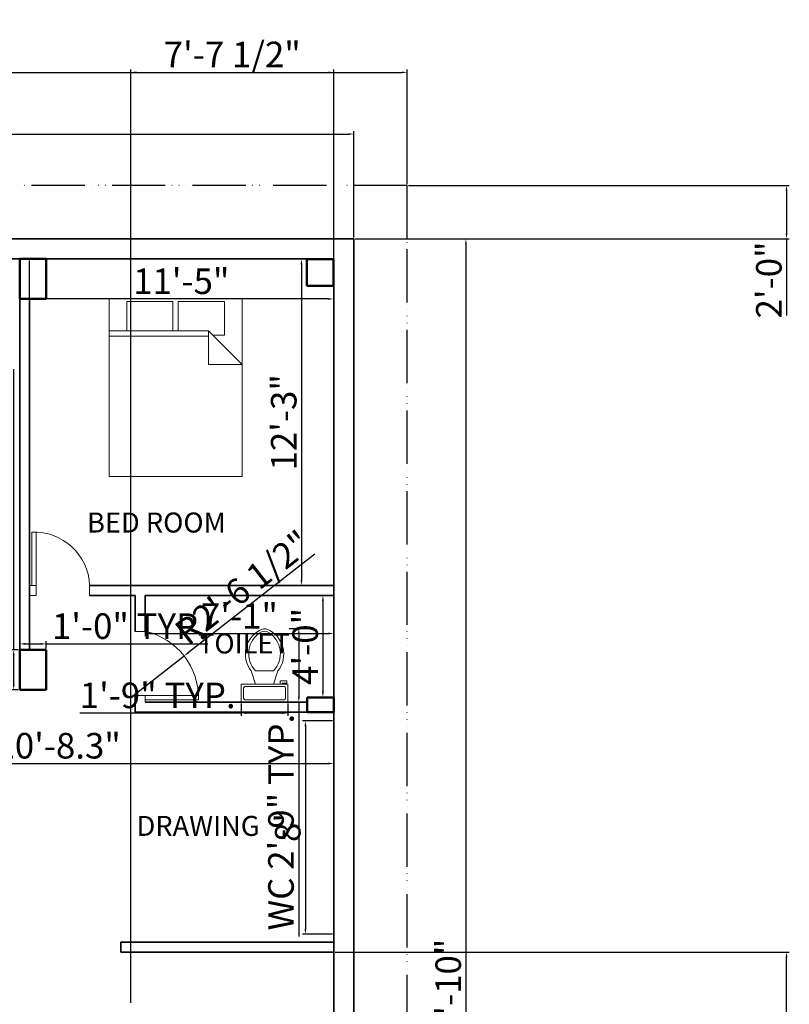
# Model space of a CAD drawing. Units: inches. Extents: x 2680 to 3617, y 1720 to 2823.
# Tile 4 of 4: x 3270 to 3617, y 2380 to 2823. Entities that reach past the tile are written whole.
import ezdxf

# ---------------------------------------------------------------- set-up
doc = ezdxf.new("R2010")
doc.units = ezdxf.units.IN
doc.linetypes.add('ACAD_ISO06W100', pattern=[36, 24, -3, 0, -3, 0, -3, 0, -3])
for name, color, linetype, lineweight in [('A-ANNO-DIMS', 2, 'Continuous', 18), ('A-AREA-IDEN', 244, 'Continuous', 18), ('A-COLS', 1, 'Continuous', 50), ('A-DOOR', 4, 'Continuous', 18), ('A-FLOR-FIXT', 9, 'Continuous', 18), ('A-FURN', 8, 'Continuous', 18), ('A-WALL', 7, 'Continuous', 35), ('C-PROP', 6, 'ACAD_ISO06W100', 25)]:
    doc.layers.add(name, color=color, linetype=linetype, lineweight=lineweight)
doc.styles.get("Standard").update_dxf_attribs({"font": 'arial.ttf'})
doc.dimstyles.new('ISO-25', dxfattribs={"dimtxt": 11.5, "dimasz": 2.5, "dimexe": 1.25, "dimexo": 0.625, "dimtad": 1, "dimdec": 1, "dimlunit": 3, "dimtxsty": 'Standard', "dimcen": 2.5, "dimadec": 0, "dimazin": 0, "dimtfac": 1, "dimtdec": 1, "dimtmove": 0, "dimatfit": 3, "dimfxl": 1, "dimarcsym": 0})

# ---------------------------------------------------------------- blocks, each defined once
blk = doc.blocks.new('*D8')
at = {"layer": 'A-ANNO-DIMS', "color": 0, "lineweight": -2, "transparency": 16777216}
for p, q in [((3274.67, 2714.72), (3274.67, 2696.18)), ((3411.72, 2714.72), (3411.72, 2696.18)), ((3409.22, 2697.43), (3277.17, 2697.43))]:
    blk.add_line(p, q, dxfattribs=at)
at = {"layer": 'A-ANNO-DIMS', "color": 0, "lineweight": 70, "transparency": 16777216}
for points in [[(3277.17, 2697.84), (3277.17, 2697.01), (3274.67, 2697.43)], [(3409.22, 2697.84), (3409.22, 2697.01), (3411.72, 2697.43)]]:
    blk.add_solid(points, dxfattribs=at)
at = {"layer": 'Defpoints', "color": 0, "lineweight": 70, "transparency": 16777216}
for p in [(3274.67, 2715.35), (3411.72, 2715.35), (3274.67, 2697.43)]:
    blk.add_point(p, dxfattribs=at)
at = {"layer": 'A-ANNO-DIMS', "color": 0, "transparency": 16777216, "insert": (3343.2, 2703.92), "char_height": 11.5, "attachment_point": 5}
blk.add_mtext('11\'-5"', dxfattribs=at)
blk = doc.blocks.new('*D9')
at = {"layer": 'A-ANNO-DIMS', "color": 0, "lineweight": -2, "transparency": 16777216}
for p, q in [((3411.29, 2715.35), (3396.09, 2715.35)), ((3397.34, 2712.85), (3397.34, 2571)), ((3411.29, 2568.5), (3396.09, 2568.5))]:
    blk.add_line(p, q, dxfattribs=at)
at = {"layer": 'A-ANNO-DIMS', "color": 0, "lineweight": 70, "transparency": 16777216}
for points in [[(3396.92, 2712.85), (3397.76, 2712.85), (3397.34, 2715.35)], [(3396.92, 2571), (3397.76, 2571), (3397.34, 2568.5)]]:
    blk.add_solid(points, dxfattribs=at)
at = {"layer": 'Defpoints', "color": 0, "lineweight": 70, "transparency": 16777216}
for p in [(3411.91, 2715.35), (3397.34, 2568.5), (3411.91, 2568.5)]:
    blk.add_point(p, dxfattribs=at)
at = {"layer": 'A-ANNO-DIMS', "color": 0, "transparency": 16777216, "insert": (3390.84, 2641.93), "char_height": 11.5, "attachment_point": 5, "rotation": 90}
blk.add_mtext('12\'-3"', dxfattribs=at)
blk = doc.blocks.new('*D12')
at = {"layer": 'A-ANNO-DIMS', "color": 0, "lineweight": -2, "transparency": 16777216}
for p, q in [((3326.91, 2563.38), (3326.91, 2545.63)), ((3411.91, 2563.38), (3411.91, 2545.63)), ((3329.41, 2546.88), (3409.41, 2546.88))]:
    blk.add_line(p, q, dxfattribs=at)
at = {"layer": 'A-ANNO-DIMS', "color": 0, "lineweight": 70, "transparency": 16777216}
for points in [[(3329.41, 2547.3), (3329.41, 2546.47), (3326.91, 2546.88)], [(3409.41, 2547.3), (3409.41, 2546.47), (3411.91, 2546.88)]]:
    blk.add_solid(points, dxfattribs=at)
at = {"layer": 'Defpoints', "color": 0, "lineweight": 70, "transparency": 16777216}
for p in [(3326.91, 2564), (3411.91, 2564), (3411.91, 2546.88)]:
    blk.add_point(p, dxfattribs=at)
at = {"layer": 'A-ANNO-DIMS', "color": 0, "transparency": 16777216, "insert": (3369.41, 2553.28), "char_height": 11.5, "attachment_point": 5}
blk.add_mtext('7\'-1"', dxfattribs=at)
blk = doc.blocks.new('*D13')
at = {"layer": 'A-ANNO-DIMS', "color": 0, "lineweight": -2, "transparency": 16777216}
for p, q in [((3411.29, 2564), (3405.73, 2564)), ((3406.98, 2561.5), (3406.98, 2520.65)), ((3411.29, 2518.15), (3405.73, 2518.15))]:
    blk.add_line(p, q, dxfattribs=at)
at = {"layer": 'A-ANNO-DIMS', "color": 0, "lineweight": 70, "transparency": 16777216}
for points in [[(3406.56, 2561.5), (3407.4, 2561.5), (3406.98, 2564)], [(3406.56, 2520.65), (3407.4, 2520.65), (3406.98, 2518.15)]]:
    blk.add_solid(points, dxfattribs=at)
at = {"layer": 'Defpoints', "color": 0, "lineweight": 70, "transparency": 16777216}
for p in [(3411.91, 2564), (3406.98, 2518.15), (3411.91, 2518.15)]:
    blk.add_point(p, dxfattribs=at)
at = {"layer": 'A-ANNO-DIMS', "color": 0, "transparency": 16777216, "insert": (3400.48, 2541.08), "char_height": 11.5, "attachment_point": 5, "rotation": 90}
blk.add_mtext('4\'-0"', dxfattribs=at)
blk = doc.blocks.new('*D14')
at = {"layer": 'A-ANNO-DIMS', "color": 0, "lineweight": -2, "transparency": 16777216}
for p, q in [((3411.29, 2507.58), (3397.87, 2507.58)), ((3399.12, 2505.08), (3399.12, 2414.04)), ((3411.29, 2411.54), (3397.87, 2411.54))]:
    blk.add_line(p, q, dxfattribs=at)
at = {"layer": 'A-ANNO-DIMS', "color": 0, "lineweight": 70, "transparency": 16777216}
for points in [[(3398.71, 2505.08), (3399.54, 2505.08), (3399.12, 2507.58)], [(3398.71, 2414.04), (3399.54, 2414.04), (3399.12, 2411.54)]]:
    blk.add_solid(points, dxfattribs=at)
at = {"layer": 'Defpoints', "color": 0, "lineweight": 70, "transparency": 16777216}
for p in [(3411.91, 2507.58), (3399.12, 2411.54), (3411.91, 2411.54)]:
    blk.add_point(p, dxfattribs=at)
at = {"layer": 'A-ANNO-DIMS', "color": 0, "transparency": 16777216, "insert": (3392.63, 2459.56), "char_height": 11.5, "attachment_point": 5, "rotation": 90}
blk.add_mtext("8'", dxfattribs=at)
blk = doc.blocks.new('*D27')
at = {"layer": 'A-ANNO-DIMS', "color": 0, "lineweight": -2, "transparency": 16777216}
for p, q in [((3163.61, 2520.88), (3163.61, 2487.12)), ((3411.91, 2517.52), (3411.91, 2487.12)), ((3166.11, 2488.37), (3409.41, 2488.37))]:
    blk.add_line(p, q, dxfattribs=at)
at = {"layer": 'A-ANNO-DIMS', "color": 0, "lineweight": 70, "transparency": 16777216}
for points in [[(3166.11, 2488.78), (3166.11, 2487.95), (3163.61, 2488.37)], [(3409.41, 2488.78), (3409.41, 2487.95), (3411.91, 2488.37)]]:
    blk.add_solid(points, dxfattribs=at)
at = {"layer": 'Defpoints', "color": 0, "lineweight": 70, "transparency": 16777216}
for p in [(3163.61, 2521.5), (3411.91, 2518.15), (3411.91, 2488.37)]:
    blk.add_point(p, dxfattribs=at)
at = {"layer": 'A-ANNO-DIMS', "color": 0, "transparency": 16777216, "insert": (3287.76, 2494.87), "char_height": 11.5, "attachment_point": 5}
blk.add_mtext('20\'-8.3"', dxfattribs=at)
blk = doc.blocks.new('*D41')
at = {"layer": 'A-ANNO-DIMS', "color": 0, "lineweight": -2, "transparency": 16777216}
for p, q in [((2888.91, 2725.13), (2888.91, 2772.91)), ((2891.41, 2771.66), (3418.41, 2771.66)), ((3420.91, 2725.13), (3420.91, 2772.91))]:
    blk.add_line(p, q, dxfattribs=at)
at = {"layer": 'A-ANNO-DIMS', "color": 0, "lineweight": 70, "transparency": 16777216}
for points in [[(2891.41, 2772.07), (2891.41, 2771.24), (2888.91, 2771.66)], [(3418.41, 2772.07), (3418.41, 2771.24), (3420.91, 2771.66)]]:
    blk.add_solid(points, dxfattribs=at)
at = {"layer": 'Defpoints', "color": 0, "lineweight": 70, "transparency": 16777216}
for p in [(3420.91, 2771.66), (2888.91, 2724.5), (3420.91, 2724.5)]:
    blk.add_point(p, dxfattribs=at)
at = {"layer": 'A-ANNO-DIMS', "color": 0, "transparency": 16777216, "insert": (3154.91, 2778.03), "char_height": 11.5, "attachment_point": 5}
blk.add_mtext('44\'-4"', dxfattribs=at)
blk = doc.blocks.new('*D43')
at = {"layer": 'A-ANNO-DIMS', "color": 0, "lineweight": -2, "transparency": 16777216}
for p, q in [((3421.54, 2724.5), (3472.64, 2724.5)), ((3471.39, 2722), (3471.39, 2045)), ((3421.54, 2042.5), (3472.64, 2042.5))]:
    blk.add_line(p, q, dxfattribs=at)
at = {"layer": 'A-ANNO-DIMS', "color": 0, "lineweight": 70, "transparency": 16777216}
for points in [[(3470.98, 2722), (3471.81, 2722), (3471.39, 2724.5)], [(3470.98, 2045), (3471.81, 2045), (3471.39, 2042.5)]]:
    blk.add_solid(points, dxfattribs=at)
at = {"layer": 'Defpoints', "color": 0, "lineweight": 70, "transparency": 16777216}
for p in [(3420.91, 2724.5), (3420.91, 2042.5), (3471.39, 2042.5)]:
    blk.add_point(p, dxfattribs=at)
at = {"layer": 'A-ANNO-DIMS', "color": 0, "transparency": 16777216, "insert": (3464.9, 2383.5), "char_height": 11.5, "attachment_point": 5, "rotation": 90}
blk.add_mtext('56\'-10"', dxfattribs=at)
blk = doc.blocks.new('Bed - Queen')
for p, q in [((0, -80.00003), (0, 0)), ((0, 0), (59.99999, 0)), ((59.99999, 0), (59.99999, -80.00003)), ((7.99999, -1.2), (28.79998, -1.2)), ((7.99999, -14.4), (7.99999, -1.2)), ((28.79998, -1.2), (28.79998, -14.4)), ((31.19999, -1.2), (51.99999, -1.2)), ((31.19999, -14.4), (31.19999, -1.2)), ((51.99999, -1.2), (51.99999, -16.4)), ((0, -14.4), (44.8, -14.4)), ((44.8, -16.8), (0, -16.8)), ((59.99999, -29.6), (44.8, -14.4)), ((44.8, -14.4), (44.8, -29.6)), ((51.99999, -16.4), (46.79936, -16.4)), ((44.8, -29.6), (59.99999, -29.6)), ((59.99999, -80.00003), (0, -80.00003))]:
    blk.add_line(p, q)
blk = doc.blocks.new('Toilet - top')
for p, q in [((9.5, -6), (9.5, -2)), ((-10, -8.5), (-8, -8.5)), ((-10, -9.5), (-10, -8.5)), ((-8, -8.5), (-8, -8)), ((-7, -8), (-7, -9.5)), ((-4, -8), (-6, -14)), ((4, -8), (6, -14)), ((-7, -9.5), (-10, -9.5)), ((4, -14), (-4, -14))]:
    blk.add_line(p, q)
blk.add_lwpolyline([(10.5, -8), (10.5, 0), (-10.5, 0), (-10.5, -8)], close=True)
for points in [[(-9.5, -2), (-9.5, -6)], [(8.5, -1), (-8.5, -1)], [(-8.5, -7), (8.5, -7)]]:
    blk.add_lwpolyline(points)
for centre, radius, start, end in [((-8.62, -1.88), 0.884, 81.8699, 188.1301), ((8.62, -1.88), 0.884, 351.8699, 98.1301), ((-8.62, -6.12), 0.884, 171.8699, 278.1301), ((8.62, -6.12), 0.884, 261.8699, 8.1301), ((3.52, -21.58), 12.17, 141.4691, 247.9714), ((4.2, -21.82), 11.33, 136.3677, 238.9468), ((-3.52, -21.58), 12.17, 292.0284, 38.5307), ((-4.2, -21.82), 11.33, 301.053, 43.6321), ((0, -27.88), 4, 245.7318, 294.2682), ((0, -29), 4, 254.8605, 285.1395)]:
    blk.add_arc(centre, radius, start, end)
blk = doc.blocks.new('COL-12X6P64')
for p, q in [((0, 0), (0, 6.64)), ((0, 6.64), (12, 6.64)), ((12, 6.64), (12, 0)), ((12, 0), (0, 0))]:
    blk.add_line(p, q)
blk = doc.blocks.new('COL-12X18')
for p, q in [((0, 0), (0, 18)), ((0, 18), (12, 18)), ((12, 18), (12, 0)), ((12, 18), (12, 0)), ((12, 0), (0, 0))]:
    blk.add_line(p, q)
blk = doc.blocks.new('COL-12X12')
for p, q in [((0, 12), (12, 12)), ((0, 0), (0, 12)), ((12, 12), (12, 0)), ((12, 0), (0, 0))]:
    blk.add_line(p, q)
blk = doc.blocks.new('DOOR-SINGLE-27')
for p, q in [((26, 28.5), (24, 28.5)), ((24, 28.5), (24, 0)), ((26, 4.5), (26, 28.5)), ((0, 4.5), (0, 0)), ((24, 4.5), (27, 4.5)), ((27, 4.5), (26, 4.5)), ((24, 0), (27, 0))]:
    blk.add_line(p, q)
blk.add_arc((25, 3.5), 25.02, 87.7094, 177.7094)
blk = doc.blocks.new('*D56')
at = {"layer": 'A-ANNO-DIMS', "color": 0, "lineweight": -2, "transparency": 16777216}
for p, q in [((3391.83, 2549.05), (3397.41, 2549.05)), ((3396.16, 2546.55), (3396.16, 2518.5)), ((3391.83, 2516), (3397.41, 2516)), ((3396.16, 2516), (3396.16, 2410.46))]:
    blk.add_line(p, q, dxfattribs=at)
at = {"layer": 'A-ANNO-DIMS', "color": 0, "lineweight": 70, "transparency": 16777216}
for points in [[(3395.74, 2546.55), (3396.58, 2546.55), (3396.16, 2549.05)], [(3395.74, 2518.5), (3396.58, 2518.5), (3396.16, 2516)]]:
    blk.add_solid(points, dxfattribs=at)
at = {"layer": 'Defpoints', "color": 0, "lineweight": 70, "transparency": 16777216}
for p in [(3391.2, 2549.05), (3391.2, 2516), (3396.16, 2516)]:
    blk.add_point(p, dxfattribs=at)
at = {"layer": 'A-ANNO-DIMS', "color": 0, "transparency": 16777216, "insert": (3389.59, 2461.98), "char_height": 11.5, "attachment_point": 5, "rotation": 90}
blk.add_mtext('WC 2\'-9" TYP.', dxfattribs=at)
blk = doc.blocks.new('*D57')
at = {"layer": 'A-ANNO-DIMS', "color": 0, "lineweight": -2, "transparency": 16777216}
for p, q in [((3370.2, 2515.38), (3370.2, 2509.8)), ((3391.2, 2515.38), (3391.2, 2509.8)), ((3370.2, 2511.05), (3297.44, 2511.05)), ((3388.7, 2511.05), (3372.7, 2511.05))]:
    blk.add_line(p, q, dxfattribs=at)
at = {"layer": 'A-ANNO-DIMS', "color": 0, "lineweight": 70, "transparency": 16777216}
for points in [[(3372.7, 2511.46), (3372.7, 2510.63), (3370.2, 2511.05)], [(3388.7, 2511.46), (3388.7, 2510.63), (3391.2, 2511.05)]]:
    blk.add_solid(points, dxfattribs=at)
at = {"layer": 'Defpoints', "color": 0, "lineweight": 70, "transparency": 16777216}
for p in [(3370.2, 2516), (3391.2, 2516), (3370.2, 2511.05)]:
    blk.add_point(p, dxfattribs=at)
at = {"layer": 'A-ANNO-DIMS', "color": 0, "transparency": 16777216, "insert": (3332.57, 2517.54), "char_height": 11.5, "attachment_point": 5}
blk.add_mtext('1\'-9" TYP.', dxfattribs=at)
blk = doc.blocks.new('*D60')
at = {"layer": 'A-ANNO-DIMS', "color": 0, "lineweight": -2, "transparency": 16777216}
for p, q in [((3267.71, 2539.5), (3267.71, 2665.89)), ((3269.79, 2539.5), (3266.46, 2539.5)), ((3267.71, 2524), (3267.71, 2537)), ((3269.79, 2521.5), (3266.46, 2521.5))]:
    blk.add_line(p, q, dxfattribs=at)
at = {"layer": 'A-ANNO-DIMS', "color": 0, "lineweight": 70, "transparency": 16777216}
for points in [[(3267.3, 2537), (3268.13, 2537), (3267.71, 2539.5)], [(3267.3, 2524), (3268.13, 2524), (3267.71, 2521.5)]]:
    blk.add_solid(points, dxfattribs=at)
at = {"layer": 'Defpoints', "color": 0, "lineweight": 70, "transparency": 16777216}
for p in [(3267.71, 2539.5), (3270.41, 2539.5), (3270.41, 2521.5)]:
    blk.add_point(p, dxfattribs=at)
at = {"layer": 'A-ANNO-DIMS', "color": 0, "transparency": 16777216, "insert": (3261.14, 2603.95), "char_height": 11.5, "attachment_point": 5, "rotation": 90}
blk.add_mtext('COL B 1\'-6" TYP.', dxfattribs=at)
blk = doc.blocks.new('*D61')
at = {"layer": 'A-ANNO-DIMS', "color": 0, "lineweight": -2, "transparency": 16777216}
for p, q in [((3270.41, 2540.13), (3270.41, 2543.45)), ((3272.91, 2542.2), (3279.91, 2542.2)), ((3282.41, 2540.13), (3282.41, 2543.45)), ((3282.41, 2542.2), (3355.18, 2542.2))]:
    blk.add_line(p, q, dxfattribs=at)
at = {"layer": 'A-ANNO-DIMS', "color": 0, "lineweight": 70, "transparency": 16777216}
for points in [[(3272.91, 2542.62), (3272.91, 2541.79), (3270.41, 2542.2)], [(3279.91, 2542.62), (3279.91, 2541.79), (3282.41, 2542.2)]]:
    blk.add_solid(points, dxfattribs=at)
at = {"layer": 'Defpoints', "color": 0, "lineweight": 70, "transparency": 16777216}
for p in [(3270.41, 2539.5), (3282.41, 2542.2), (3282.41, 2539.5)]:
    blk.add_point(p, dxfattribs=at)
at = {"layer": 'A-ANNO-DIMS', "color": 0, "transparency": 16777216, "insert": (3320.05, 2548.7), "char_height": 11.5, "attachment_point": 5}
blk.add_mtext('1\'-0" TYP.', dxfattribs=at)
blk = doc.blocks.new('*D68')
at = {"layer": 'A-ANNO-DIMS', "color": 0, "lineweight": -2, "transparency": 16777216}
for p, q in [((2864.91, 2749.13), (2864.91, 2800.65)), ((3444.91, 2749.13), (3444.91, 2800.65)), ((2867.41, 2799.4), (3442.41, 2799.4))]:
    blk.add_line(p, q, dxfattribs=at)
at = {"layer": 'A-ANNO-DIMS', "color": 0, "lineweight": 70, "transparency": 16777216}
for points in [[(2867.41, 2799.82), (2867.41, 2798.99), (2864.91, 2799.4)], [(3442.41, 2799.82), (3442.41, 2798.99), (3444.91, 2799.4)]]:
    blk.add_solid(points, dxfattribs=at)
at = {"layer": 'Defpoints', "color": 0, "lineweight": 70, "transparency": 16777216}
for p in [(3444.91, 2799.4), (2864.91, 2748.5), (3444.91, 2748.5)]:
    blk.add_point(p, dxfattribs=at)
at = {"layer": 'A-ANNO-DIMS', "color": 0, "transparency": 16777216, "insert": (3154.91, 2805.9), "char_height": 11.5, "attachment_point": 5}
blk.add_mtext('48\'-4"', dxfattribs=at)
blk = doc.blocks.new('*D72')
at = {"layer": 'A-ANNO-DIMS', "color": 0, "lineweight": -2, "transparency": 16777216}
for p, q in [((3445.54, 2748.5), (3617.06, 2748.5)), ((3615.81, 2746), (3615.81, 2727)), ((3421.54, 2724.5), (3617.06, 2724.5)), ((3615.81, 2724.5), (3615.81, 2689.99))]:
    blk.add_line(p, q, dxfattribs=at)
at = {"layer": 'A-ANNO-DIMS', "color": 0, "lineweight": 70, "transparency": 16777216}
for points in [[(3615.4, 2746), (3616.23, 2746), (3615.81, 2748.5)], [(3615.4, 2727), (3616.23, 2727), (3615.81, 2724.5)]]:
    blk.add_solid(points, dxfattribs=at)
at = {"layer": 'Defpoints', "color": 0, "lineweight": 70, "transparency": 16777216}
for p in [(3444.91, 2748.5), (3420.91, 2724.5), (3615.81, 2724.5)]:
    blk.add_point(p, dxfattribs=at)
at = {"layer": 'A-ANNO-DIMS', "color": 0, "transparency": 16777216, "insert": (3609.32, 2706), "char_height": 11.5, "attachment_point": 5, "rotation": 90}
blk.add_mtext('2\'-0"', dxfattribs=at)
blk = doc.blocks.new('*D73')
at = {"layer": 'A-ANNO-DIMS', "color": 0, "lineweight": -2, "transparency": 16777216}
for p, q in [((3320.41, 2380.61), (3320.41, 2800.65)), ((3411.91, 2404.13), (3411.91, 2800.65)), ((3322.91, 2799.4), (3409.41, 2799.4))]:
    blk.add_line(p, q, dxfattribs=at)
at = {"layer": 'A-ANNO-DIMS', "color": 0, "lineweight": 70, "transparency": 16777216}
for points in [[(3322.91, 2799.82), (3322.91, 2798.99), (3320.41, 2799.4)], [(3409.41, 2799.82), (3409.41, 2798.99), (3411.91, 2799.4)]]:
    blk.add_solid(points, dxfattribs=at)
at = {"layer": 'Defpoints', "color": 0, "lineweight": 70, "transparency": 16777216}
for p in [(3411.91, 2799.4), (3411.91, 2403.5), (3320.41, 2379.98)]:
    blk.add_point(p, dxfattribs=at)
at = {"layer": 'A-ANNO-DIMS', "color": 0, "transparency": 16777216, "insert": (3366.16, 2805.98), "char_height": 11.5, "attachment_point": 5}
blk.add_mtext('7\'-7 1/2"', dxfattribs=at)
blk = doc.blocks.new('*D74')
at = {"layer": 'A-ANNO-DIMS', "color": 0, "lineweight": -2, "transparency": 16777216}
for p, q in [((3412.54, 2403.5), (3617.06, 2403.5)), ((3615.81, 2310), (3615.81, 2401)), ((3321.04, 2307.5), (3617.06, 2307.5))]:
    blk.add_line(p, q, dxfattribs=at)
at = {"layer": 'A-ANNO-DIMS', "color": 0, "lineweight": 70, "transparency": 16777216}
for points in [[(3615.4, 2401), (3616.23, 2401), (3615.81, 2403.5)], [(3615.4, 2310), (3616.23, 2310), (3615.81, 2307.5)]]:
    blk.add_solid(points, dxfattribs=at)
at = {"layer": 'Defpoints', "color": 0, "lineweight": 70, "transparency": 16777216}
for p in [(3411.91, 2403.5), (3615.81, 2403.5), (3320.41, 2307.5)]:
    blk.add_point(p, dxfattribs=at)
at = {"layer": 'A-ANNO-DIMS', "color": 0, "transparency": 16777216, "insert": (3609.32, 2355.5), "char_height": 11.5, "attachment_point": 5, "rotation": 90}
blk.add_mtext('8\'-0"', dxfattribs=at)
blk = doc.blocks.new('*D75')
at = {"layer": 'A-ANNO-DIMS', "color": 0, "lineweight": -2, "transparency": 16777216}
for p, q in [((3403.37, 2582.6), (3346.46, 2538.29)), ((3320.41, 2518), (3344.49, 2536.76))]:
    blk.add_line(p, q, dxfattribs=at)
at = {"layer": 'A-ANNO-DIMS', "color": 0, "lineweight": 70, "transparency": 16777216}
blk.add_solid([(3346.21, 2538.62), (3346.72, 2537.96), (3344.49, 2536.76)], dxfattribs=at)
at = {"layer": 'Defpoints', "color": 0, "lineweight": 70, "transparency": 16777216}
for p in [(3344.49, 2536.76), (3320.41, 2518)]:
    blk.add_point(p, dxfattribs=at)
at = {"layer": 'A-ANNO-DIMS', "color": 0, "transparency": 16777216, "insert": (3371.87, 2566.4), "char_height": 11.5, "attachment_point": 5, "rotation": 37.9058}
blk.add_mtext('R2\'-6 1/2"', dxfattribs=at)

msp = doc.modelspace()

# ---------------------------------------------------------------- linework, layer by layer
at = {"layer": 'A-DOOR'}
for p, q in [((3322.41, 2547.83), (3326.91, 2547.83)), ((3350.91, 2519), (3322.41, 2519)), ((3326.91, 2519), (3326.91, 2516)), ((3350.91, 2517), (3350.91, 2519)), ((3326.91, 2516), (3326.91, 2517)), ((3326.91, 2517), (3350.91, 2517)), ((3326.91, 2516), (3326.91, 2516))]:
    msp.add_line(p, q, dxfattribs=at)
msp.add_arc((3320.41, 2518), 30.52, 358.1226, 77.6899, dxfattribs=at)
at = {"layer": 'A-WALL'}
for p, q in [((2888.91, 2724.5), (3420.91, 2724.5)), ((3420.91, 2724.5), (3420.91, 2086)), ((2897.91, 2715.5), (3411.91, 2715.5)), ((3270.41, 2715.5), (3270.41, 2521.5)), ((3274.91, 2715.5), (3274.91, 2715.43)), ((3411.91, 2715.5), (3411.91, 2086)), ((3274.91, 2697.43), (3274.91, 2539.5)), ((3301.91, 2568.5), (3411.91, 2568.5)), ((3301.91, 2564), (3322.41, 2564)), ((3322.41, 2564), (3322.41, 2547.83)), ((3326.91, 2564), (3326.91, 2547.83)), ((3326.91, 2564), (3411.91, 2564)), ((3274.91, 2539.58), (3274.91, 2539.5)), ((3270.41, 2521.5), (3274.91, 2521.5)), ((3322.41, 2519), (3322.41, 2511.5)), ((3326.91, 2516), (3399.91, 2516)), ((3322.41, 2511.5), (3411.91, 2511.5)), ((3315.91, 2408), (3411.91, 2408)), ((3315.91, 2408), (3349.5, 2408)), ((3315.91, 2408), (3315.91, 2403.5)), ((3315.91, 2403.5), (3411.91, 2403.5))]:
    msp.add_line(p, q, dxfattribs=at)
at = {"layer": 'C-PROP'}
for p, q in [((3444.91, 2748.5), (2888.91, 2748.5)), ((3444.91, 2724.5), (3444.91, 2748.5)), ((3444.91, 2042.5), (3444.91, 2724.5))]:
    msp.add_line(p, q, dxfattribs=at)

# ---------------------------------------------------------------- block references
at = {"layer": 'A-COLS'}
for name, p in [('COL-12X18', (3270.41, 2697.43)), ('COL-12X12', (3399.72, 2703.35)), ('COL-12X18', (3270.41, 2521.5)), ('COL-12X6P64', (3399.91, 2511.5))]:
    msp.add_blockref(name, p, dxfattribs=at)
at = {"layer": 'A-DOOR', "extrusion": (0, 0, -1), "zscale": -1}
msp.add_blockref('DOOR-SINGLE-27', (-3301.91, 2564), dxfattribs=at)
at = {"layer": 'A-FLOR-FIXT', "rotation": 180}
msp.add_blockref('Toilet - top', (3380.7, 2516), dxfattribs=at)
at = {"layer": 'A-FURN'}
msp.add_blockref('Bed - Queen', (3310.67, 2697.52), dxfattribs=at)

# ---------------------------------------------------------------- texts
at = {"layer": 'A-AREA-IDEN', "char_height": 9, "attachment_point": 1}
for s, insert in [('{BED ROOM}', (3300.75, 2601.32)), ('{TOILET}', (3350.76, 2546.88)), ('{DRAWING}', (3323.04, 2464.78))]:
    msp.add_mtext_dynamic_manual_height_columns(s, width=87.2951, gutter_width=12.5, heights=[0], dxfattribs=dict(at, insert=insert))

# ---------------------------------------------------------------- dimensions: what is measured, and where the dimension line sits
at = {"layer": 'A-ANNO-DIMS'}
for base, p1, p2, override, picture, middle in [((3411.91, 2799.4), (3320.41, 2379.98), (3411.91, 2403.5), {"dimdec": 1, "dimlfac": 1, "dimrnd": 0, "dimzin": 1, "dimdsep": 46, "dimlunit": 4, "dimfrac": 2}, '*D73', (3366.16, 2805.98)), ((3444.91, 2799.4), (2864.91, 2748.5), (3444.91, 2748.5), {"dimdec": 1, "dimlfac": 1, "dimrnd": 0, "dimzin": 1, "dimdsep": 46, "dimlunit": 4, "dimfrac": 2}, '*D68', (3154.91, 2805.9)), ((3420.91, 2771.66), (2888.91, 2724.5), (3420.91, 2724.5), {"dimclrd": 0, "dimclre": 0, "dimclrt": 0}, '*D41', (3154.91, 2778.03)), ((3274.6746, 2697.4268), (3411.7202, 2715.349), (3274.6746, 2715.349), {"dimclrd": 0, "dimclre": 0, "dimclrt": 0}, '*D8', (3343.1974, 2703.9233)), ((3411.91, 2546.88), (3326.91, 2564), (3411.91, 2564), {"dimclrd": 0, "dimclre": 0, "dimclrt": 0}, '*D12', (3369.41, 2553.28)), ((3411.91, 2488.37), (3163.61, 2521.5), (3411.91, 2518.15), {"dimclrd": 0, "dimclre": 0, "dimclrt": 0}, '*D27', (3287.76, 2494.87))]:
    dim = msp.add_linear_dim(base=base, p1=p1, p2=p2, dimstyle='ISO-25', override=override, dxfattribs=at)
    dim.commit()
    dim.dimension.update_dxf_attribs({"geometry": picture, "text_midpoint": middle})
for base, p1, p2, override, picture, middle in [((3615.81, 2724.5), (3444.91, 2748.5), (3420.91, 2724.5), {"dimdec": 1, "dimlfac": 1, "dimrnd": 0, "dimzin": 1, "dimdsep": 46, "dimlunit": 4, "dimfrac": 2}, '*D72', (3609.32, 2706)), ((3471.39, 2042.5), (3420.91, 2724.5), (3420.91, 2042.5), {"dimclrd": 0, "dimclre": 0, "dimclrt": 0}, '*D43', (3464.9, 2383.5)), ((3399.12, 2411.54), (3411.91, 2507.58), (3411.91, 2411.54), {"dimclrd": 0, "dimclre": 0, "dimclrt": 0}, '*D14', (3392.63, 2459.56)), ((3615.81, 2403.5), (3320.41, 2307.5), (3411.91, 2403.5), {"dimdec": 1, "dimlfac": 1, "dimrnd": 0, "dimzin": 1, "dimdsep": 46, "dimlunit": 4, "dimfrac": 2}, '*D74', (3609.32, 2355.5))]:
    dim = msp.add_linear_dim(base=base, p1=p1, p2=p2, angle=90, dimstyle='ISO-25', override=override, dxfattribs=at)
    dim.commit()
    dim.dimension.update_dxf_attribs({"geometry": picture, "text_midpoint": middle})
for base, p1, p2, angle, text, override, picture, middle in [((3397.34, 2568.5), (3411.91, 2715.35), (3411.91, 2568.5), 90, '12\'-3"', {"dimclrd": 0, "dimclre": 0, "dimclrt": 0}, '*D9', (3390.84, 2641.93)), ((3267.71, 2539.5), (3270.41, 2521.5), (3270.41, 2539.5), 90, 'COL B <> TYP.', {"dimdec": 1, "dimlfac": 1, "dimrnd": 0, "dimzin": 1, "dimdsep": 46, "dimlunit": 4, "dimfrac": 2}, '*D60', (3261.14, 2603.95)), ((3406.98, 2518.15), (3411.91, 2564), (3411.91, 2518.15), 90, '4\'-0"', {"dimclrd": 0, "dimclre": 0, "dimclrt": 0}, '*D13', (3400.48, 2541.08)), ((3396.161, 2516.0039), (3391.2041, 2549.0502), (3391.2041, 2516.0039), 270, 'WC <> TYP.', {"dimdec": 1, "dimlfac": 1, "dimrnd": 0, "dimzin": 1, "dimdsep": 46, "dimlunit": 4, "dimfrac": 2}, '*D56', (3389.5899, 2461.98)), ((3370.2, 2511.05), (3391.2, 2516), (3370.2, 2516), 180, '<> TYP.', {"dimdec": 1, "dimlfac": 1, "dimrnd": 0, "dimzin": 1, "dimdsep": 46, "dimlunit": 4, "dimfrac": 2}, '*D57', (3332.57, 2517.54))]:
    dim = msp.add_linear_dim(base=base, p1=p1, p2=p2, angle=angle, text=text, dimstyle='ISO-25', override=override, dxfattribs=at)
    dim.commit()
    dim.dimension.update_dxf_attribs({"geometry": picture, "text_midpoint": middle})
dim = msp.add_radius_dim(center=(3320.41, 2518), mpoint=(3344.49, 2536.76), dimstyle='ISO-25', override={"dimdec": 1, "dimlfac": 1, "dimrnd": 0, "dimzin": 1, "dimdsep": 46, "dimlunit": 4, "dimfrac": 2}, dxfattribs=at)
dim.commit()
dim.dimension.update_dxf_attribs({"geometry": '*D75', "text_midpoint": (3371.87, 2566.4)})
dim = msp.add_linear_dim(base=(3282.41, 2542.2), p1=(3270.41, 2539.5), p2=(3282.41, 2539.5), text='<> TYP.', dimstyle='ISO-25', override={"dimdec": 1, "dimlfac": 1, "dimrnd": 0, "dimzin": 1, "dimdsep": 46, "dimlunit": 4, "dimfrac": 2}, dxfattribs=at)
dim.commit()
dim.dimension.update_dxf_attribs({"geometry": '*D61', "text_midpoint": (3320.05, 2548.7)})

doc.saveas('drawing.dxf')
